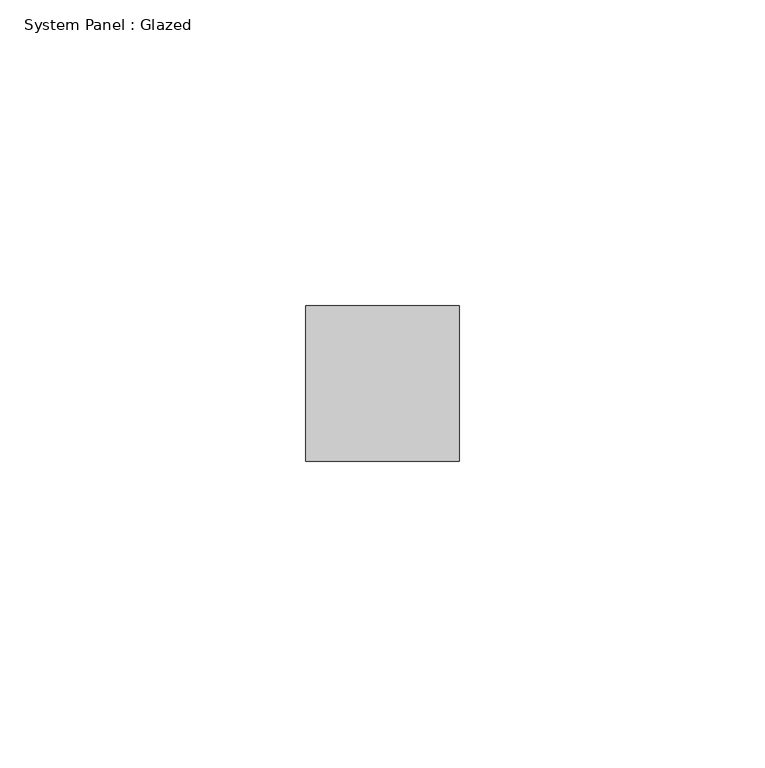
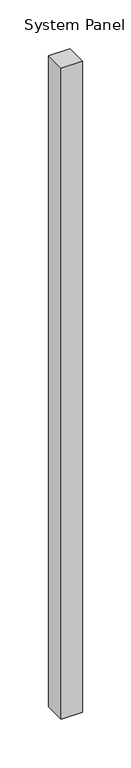
"""IFC4 building model written with IfcOpenShell, lengths in millimetres: plate geometry, System Panel : Glazed."""

from ifc_helpers import new_model, si_unit, origin, origin_with_axes, place, context, project, spatial, polyline, outline, extrude, source, transform, mapped, element, save


def system_panel_glazed_2cc39d43(model_context):
    return source(origin(), model_context, "Body", "SweptSolid", [
        extrude(outline(polyline([(12.5253346, 19.05), (-12.5253346, 19.05), (-12.5253346, 44.45), (12.5253346, 44.45), (12.5253346, 19.05)])), origin_with_axes(), (0.0, 0.0, 1.0), 812.8),
    ])


if __name__ == "__main__":
    model = new_model("IFC4")
    model_context = context("Model", 3, world=origin())
    ifc_project = project(units=[si_unit("LENGTHUNIT", "METRE", prefix="MILLI")], contexts=[model_context])
    site = spatial("IfcSite", under=ifc_project)
    building = spatial("IfcBuilding", under=site)
    placement = place(None, origin())
    system_panel_glazed_shape = system_panel_glazed_2cc39d43(model_context)
    element("IfcPlate", 1, ObjectType="System Panel : Glazed", at=placement, inside=building, context=model_context, shape_type="MappedRepresentation", body=[
        mapped(system_panel_glazed_shape, transform((0.0, 0.0, 0.0), x_axis=(1.0, 0.0, 0.0), y_axis=(0.0, 1.0, 0.0), z_axis=(0.0, 0.0, 1.0))),
    ])
    save(model, "model.ifc")

# Revit data of these elements
# Type "System Panel : Glazed"
#   Construction Type Id = "GSP4R"
#   Analytic Construction = "1/8 in Pilkington single glazing"
#   Visual Light Transmittance = 0.9
#   Solar Heat Gain Coefficient = 0.86
#   Heat Transfer Coefficient (U) = 1.18115 BTU/(h·ft²·°F)
# Element 1 (IfcPlate, "System Panel : Glazed")
#   Materials on its faces: "Glass"
# Materials
#   "Glass": class "Glass", colour RGB 0 128 192, transparency 0.75, Description = "Soda Lime Glass", Cost = 0
